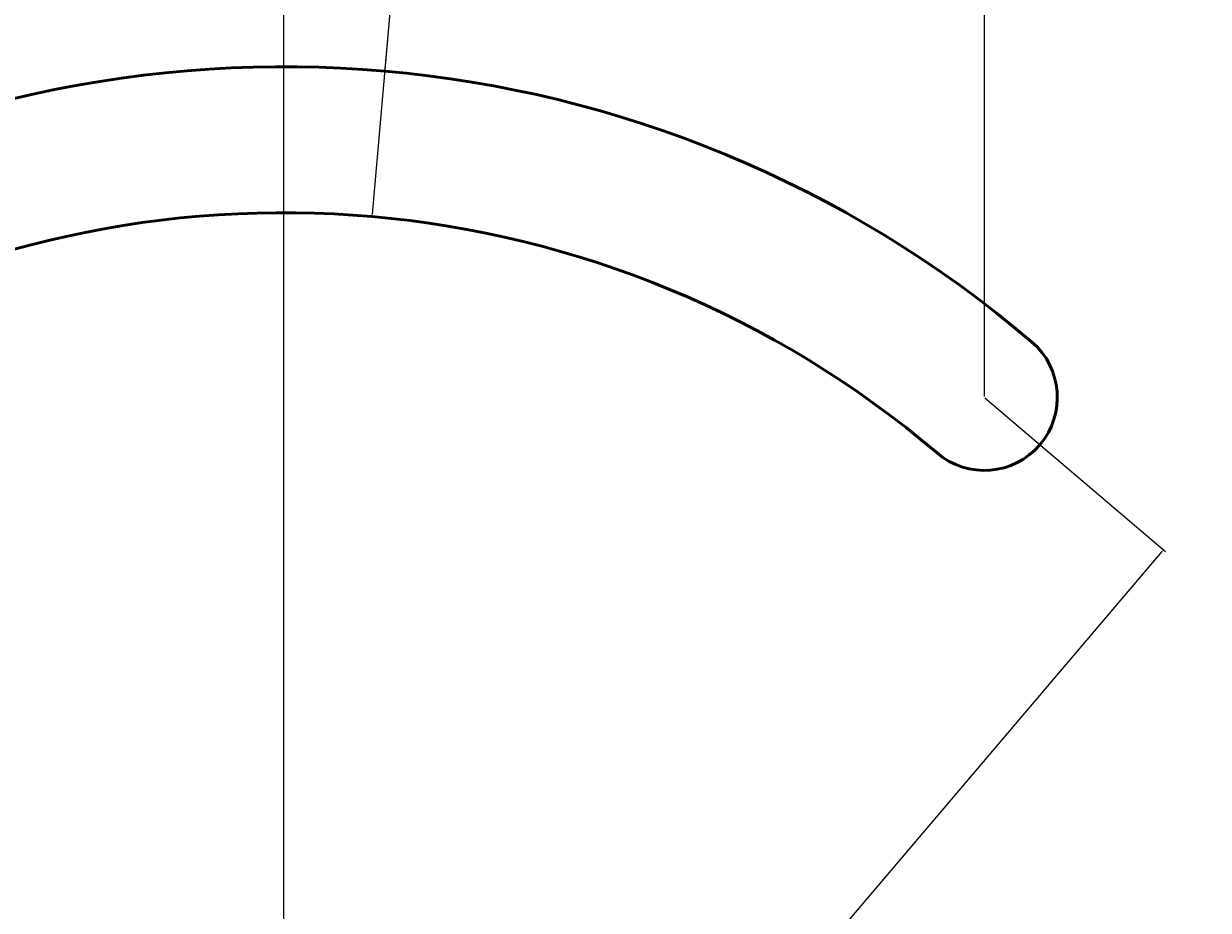
# Model space of a CAD drawing. Units: inches. Extents: x 457 to 775, y 319 to 541.
# Tile 6 of 12: x 536 to 623, y 385 to 450. Entities that reach past the tile are written whole.
import ezdxf

# ---------------------------------------------------------------- set-up
doc = ezdxf.new("R2010")
doc.units = ezdxf.units.IN
doc.header["$MEASUREMENT"] = 0
doc.layers.add('M-DIMS', color=2, linetype='Continuous', lineweight=18)
doc.layers.add('M-OUTL', color=7, linetype='Continuous', lineweight=50)
doc.styles.get("Standard").update_dxf_attribs({"font": 'arial.ttf'})
doc.dimstyles.get("Standard").update_dxf_attribs({"dimtxt": 0.18, "dimasz": 0.18, "dimexe": 0.18, "dimexo": 0.0625, "dimgap": 0.09, "dimtad": 0, "dimtih": 1, "dimtoh": 1, "dimdec": 4, "dimzin": 0, "dimdsep": 46, "dimtxsty": 'Standard', "dimcen": 0.09, "dimadec": 0, "dimazin": 0, "dimtfac": 1, "dimtdec": 4, "dimtofl": 0, "dimtmove": 0, "dimatfit": 3, "dimfxl": 1, "dimtolj": 1, "dimtzin": 0, "dimarcsym": 0})

# ---------------------------------------------------------------- blocks, each defined once
blk = doc.blocks.new('*D3')
at = {"layer": 'Defpoints', "color": 0, "transparency": 16777216}
for p in [(456.906, 523.213), (646.001, 523.213), (474.306, 336.696)]:
    blk.add_point(p, dxfattribs=at)
at = {"layer": 'M-DIMS', "color": 0, "lineweight": -2, "transparency": 16777216}
for p, q in [((645.939, 523.213), (456.726, 523.213)), ((456.906, 523.033), (456.906, 430.136)), ((456.906, 336.876), (456.906, 429.773)), ((474.244, 336.696), (456.726, 336.696))]:
    blk.add_line(p, q, dxfattribs=at)
at = {"layer": 'M-DIMS', "color": 0, "transparency": 16777216}
for points in [[(456.876, 523.033), (456.936, 523.033), (456.906, 523.213)], [(456.876, 336.876), (456.936, 336.876), (456.906, 336.696)]]:
    blk.add_solid(points, dxfattribs=at)
at = {"layer": 'M-DIMS', "color": 0, "transparency": 16777216, "insert": (456.906, 429.954), "char_height": 0.18, "attachment_point": 5}
blk.add_mtext('\\A1;186.5', dxfattribs=at)
blk = doc.blocks.new('*D16')
at = {"layer": 'Defpoints', "color": 0, "transparency": 16777216}
for p in [(554.931, 540.613), (514.502, 430.729), (554.931, 361.696)]:
    blk.add_point(p, dxfattribs=at)
at = {"layer": 'M-DIMS', "color": 0, "lineweight": -2, "transparency": 16777216}
for p, q in [((514.502, 430.791), (514.502, 540.793)), ((554.931, 361.759), (554.931, 540.793)), ((514.682, 540.613), (534.319, 540.613)), ((554.751, 540.613), (535.114, 540.613))]:
    blk.add_line(p, q, dxfattribs=at)
at = {"layer": 'M-DIMS', "color": 0, "transparency": 16777216}
for points in [[(514.682, 540.643), (514.682, 540.583), (514.502, 540.613)], [(554.751, 540.643), (554.751, 540.583), (554.931, 540.613)]]:
    blk.add_solid(points, dxfattribs=at)
at = {"layer": 'M-DIMS', "color": 0, "transparency": 16777216, "insert": (534.716, 540.613), "char_height": 0.18, "attachment_point": 5}
blk.add_mtext('\\A1;40.43', dxfattribs=at)
blk = doc.blocks.new('*D17')
at = {"layer": 'Defpoints', "color": 0, "transparency": 16777216}
for p in [(606.761, 540.613), (606.761, 422.636), (554.931, 361.696)]:
    blk.add_point(p, dxfattribs=at)
at = {"layer": 'M-DIMS', "color": 0, "lineweight": -2, "transparency": 16777216}
for p, q in [((554.931, 361.759), (554.931, 540.793)), ((606.761, 422.698), (606.761, 540.793)), ((555.111, 540.613), (580.452, 540.613)), ((606.581, 540.613), (581.24, 540.613))]:
    blk.add_line(p, q, dxfattribs=at)
at = {"layer": 'M-DIMS', "color": 0, "transparency": 16777216}
for points in [[(555.111, 540.643), (555.111, 540.583), (554.931, 540.613)], [(606.581, 540.643), (606.581, 540.583), (606.761, 540.613)]]:
    blk.add_solid(points, dxfattribs=at)
at = {"layer": 'M-DIMS', "color": 0, "transparency": 16777216, "insert": (580.846, 540.613), "char_height": 0.18, "attachment_point": 5}
blk.add_mtext('\\A1;51.83', dxfattribs=at)
blk = doc.blocks.new('*D18')
at = {"layer": 'Defpoints', "color": 0, "transparency": 16777216}
for p in [(606.761, 422.636), (554.931, 361.696), (568.185, 350.423)]:
    blk.add_point(p, dxfattribs=at)
at = {"layer": 'M-DIMS', "color": 0, "lineweight": -2, "transparency": 16777216}
for p, q in [((606.809, 422.595), (620.153, 411.246)), ((619.899, 411.226), (594.255, 381.075)), ((568.302, 350.56), (593.946, 380.711)), ((554.979, 361.656), (568.323, 350.306))]:
    blk.add_line(p, q, dxfattribs=at)
at = {"layer": 'M-DIMS', "color": 0, "transparency": 16777216}
for points in [[(619.876, 411.245), (619.922, 411.206), (620.015, 411.363)], [(568.279, 350.58), (568.325, 350.541), (568.185, 350.423)]]:
    blk.add_solid(points, dxfattribs=at)
at = {"layer": 'M-DIMS', "color": 0, "transparency": 16777216, "insert": (594.1, 380.893), "char_height": 0.18, "attachment_point": 5}
blk.add_mtext('\\A1;80', dxfattribs=at)
blk = doc.blocks.new('*D19')
at = {"layer": 'Defpoints', "color": 0, "transparency": 16777216}
for p in [(562.393, 446.769), (554.931, 361.696)]:
    blk.add_point(p, dxfattribs=at)
at = {"layer": 'M-DIMS', "color": 0, "lineweight": -2, "transparency": 16777216}
for p, q in [((566.87, 497.813), (562.409, 446.949)), ((567.05, 497.813), (566.87, 497.813)), ((554.841, 361.696), (555.021, 361.696)), ((554.931, 361.606), (554.931, 361.786))]:
    blk.add_line(p, q, dxfattribs=at)
at = {"layer": 'M-DIMS', "color": 0, "transparency": 16777216}
blk.add_solid([(562.379, 446.951), (562.439, 446.946), (562.393, 446.769)], dxfattribs=at)
at = {"layer": 'M-DIMS', "color": 0, "transparency": 16777216, "insert": (567.46, 497.813), "char_height": 0.18, "attachment_point": 5}
blk.add_mtext('\\A1;R85.4', dxfattribs=at)
blk = doc.blocks.new('*D20')
at = {"layer": 'Defpoints', "color": 0, "transparency": 16777216}
for p in [(561.45, 436.011), (554.931, 361.696)]:
    blk.add_point(p, dxfattribs=at)
at = {"layer": 'M-DIMS', "color": 0, "lineweight": -2, "transparency": 16777216}
for p, q in [((565.361, 480.599), (561.466, 436.19)), ((565.541, 480.599), (565.361, 480.599)), ((554.841, 361.696), (555.021, 361.696)), ((554.931, 361.606), (554.931, 361.786))]:
    blk.add_line(p, q, dxfattribs=at)
at = {"layer": 'M-DIMS', "color": 0, "transparency": 16777216}
blk.add_solid([(561.436, 436.193), (561.496, 436.187), (561.45, 436.011)], dxfattribs=at)
at = {"layer": 'M-DIMS', "color": 0, "transparency": 16777216, "insert": (565.951, 480.599), "char_height": 0.18, "attachment_point": 5}
blk.add_mtext('\\A1;R74.6', dxfattribs=at)

msp = doc.modelspace()

# ---------------------------------------------------------------- linework, layer by layer
at = {"layer": 'M-OUTL'}
for centre, radius, start, end in [((554.931, 361.696), 85.4, 49.61848, 120.35555), ((554.931, 361.696), 74.6, 49.61848, 120.35555), ((606.761, 422.636), 5.4, 229.61848, 49.61848)]:
    msp.add_arc(centre, radius, start, end, dxfattribs=at)

# ---------------------------------------------------------------- dimensions: what is measured, and where the dimension line sits
at = {"layer": 'M-DIMS'}
for base, p1, p2, picture, middle in [((554.931, 540.613), (514.502, 430.729), (554.931, 361.696), '*D16', (534.716, 540.613)), ((606.761, 540.613), (554.931, 361.696), (606.761, 422.636), '*D17', (580.846, 540.613))]:
    dim = msp.add_linear_dim(base=base, p1=p1, p2=p2, dimstyle='Standard', override={"dimdec": 2, "dimlfac": 1, "dimrnd": 0, "dimzin": 0, "dimdsep": 46, "dimlunit": 2}, dxfattribs=at)
    dim.commit()
    dim.dimension.update_dxf_attribs({"geometry": picture, "text_midpoint": middle})
for base, p1, p2, angle, override, picture, middle in [((456.906, 523.213), (474.306, 336.696), (646.001, 523.213), 90, {"dimdec": 1, "dimlfac": 1, "dimrnd": 0, "dimzin": 0, "dimdsep": 46, "dimlunit": 2}, '*D3', (456.906, 429.954)), ((568.185, 350.423), (606.761, 422.636), (554.931, 361.696), 229.61848, {"dimdec": 0, "dimlfac": 1, "dimrnd": 0, "dimzin": 0, "dimdsep": 46, "dimlunit": 2}, '*D18', (594.1, 380.893))]:
    dim = msp.add_linear_dim(base=base, p1=p1, p2=p2, angle=angle, dimstyle='Standard', override=override, dxfattribs=at)
    dim.commit()
    dim.dimension.update_dxf_attribs({"geometry": picture, "text_midpoint": middle})
for mpoint, picture, middle in [((562.393, 446.769), '*D19', (567.46, 497.813)), ((561.45, 436.011), '*D20', (565.951, 480.599))]:
    dim = msp.add_radius_dim(center=(554.931, 361.696), mpoint=mpoint, dimstyle='Standard', override={"dimdec": 1, "dimlfac": 1, "dimrnd": 0, "dimzin": 0, "dimdsep": 46, "dimlunit": 2}, dxfattribs=at)
    dim.commit()
    dim.dimension.update_dxf_attribs({"geometry": picture, "text_midpoint": middle, "dimtype": 164})

doc.saveas('drawing.dxf')
